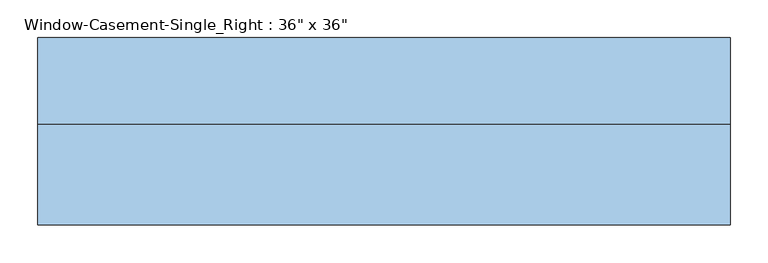
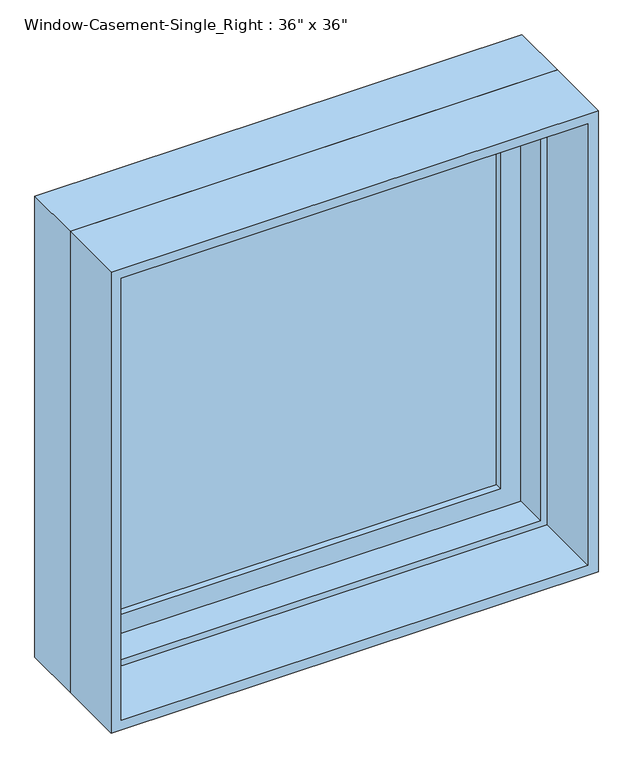
"""IFC4 building model written with IfcOpenShell, lengths in millimetres: window geometry."""

from ifc_helpers import new_model, si_unit, frame, origin, place, context, project, spatial, polyline, outline, extrude, faceted_brep, source, transform, mapped, element, save


def window_df0b8b67(model_context):
    return source(origin(), model_context, "Body", "SolidModel", [
        faceted_brep([(425.45, 82.55, 1797.05), (425.45, 19.05, 1797.05), (-425.45, 19.05, 1797.05), (-425.45, 82.55, 1797.05), (444.5, 133.35, 1816.1), (444.5, 82.55, 1816.1), (-444.5, 82.55, 1816.1), (-444.5, 133.35, 1816.1), (457.2, 19.05, 1828.8), (457.2, 133.35, 1828.8), (-457.2, 133.35, 1828.8), (-457.2, 19.05, 1828.8), (-425.45, 19.05, 946.15), (-425.45, 82.55, 946.15), (-444.5, 82.55, 927.1), (-444.5, 133.35, 927.1), (-457.2, 133.35, 914.4), (-457.2, 19.05, 914.4), (425.45, 19.05, 946.15), (425.45, 82.55, 946.15), (444.5, 82.55, 927.1), (444.5, 133.35, 927.1), (457.2, 133.35, 914.4), (457.2, 19.05, 914.4)], [[[0, 1, 2, 3]], [[4, 5, 6, 7]], [[8, 9, 10, 11]], [[3, 2, 12, 13]], [[7, 6, 14, 15]], [[11, 10, 16, 17]], [[13, 12, 18, 19]], [[15, 14, 20, 21]], [[17, 16, 22, 23]], [[11, 17, 23, 8], [1, 18, 12, 2]], [[19, 18, 1, 0]], [[5, 20, 14, 6], [3, 13, 19, 0]], [[21, 20, 5, 4]], [[23, 22, 9, 8]], [[9, 22, 16, 10], [7, 15, 21, 4]]]),
        extrude(outline(polyline([(1828.8, -457.2), (914.4, -457.2), (914.4, 457.2), (1828.8, 457.2), (1828.8, -457.2)]), holes=[polyline([(1809.75, 438.15), (933.45, 438.15), (933.45, -438.15), (1809.75, -438.15), (1809.75, 438.15)])]), frame((0.0, -114.3, 0.0), z_axis=(0.0, 1.0, 0.0), x_axis=(0.0, 0.0, 1.0)), (0.0, 0.0, 1.0), 133.35),
        extrude(outline(polyline([(1816.1, -444.5), (927.1, -444.5), (927.1, 444.5), (1816.1, 444.5), (1816.1, -444.5)]), holes=[polyline([(1758.95, 387.35), (984.25, 387.35), (984.25, -387.35), (1758.95, -387.35), (1758.95, 387.35)])]), frame((0.0, 82.55, 0.0), z_axis=(0.0, 1.0, 0.0), x_axis=(0.0, 0.0, 1.0)), (0.0, 0.0, 1.0), 44.45),
        extrude(outline(polyline([(387.35, 114.3), (387.35, 107.95), (-387.35, 107.95), (-387.35, 114.3), (387.35, 114.3)])), frame((0.0, 0.0, 984.25), z_axis=(0.0, 0.0, 1.0), x_axis=(1.0, 0.0, 0.0)), (0.0, 0.0, 1.0), 774.7),
        extrude(outline(polyline([(-387.35, 95.25), (-387.35, 101.6), (387.35, 101.6), (387.35, 95.25), (-387.35, 95.25)])), frame((0.0, 0.0, 984.25), z_axis=(0.0, 0.0, 1.0), x_axis=(1.0, 0.0, 0.0)), (0.0, 0.0, 1.0), 774.7),
    ])


if __name__ == "__main__":
    model = new_model("IFC4")
    model_context = context("Model", 3, world=origin())
    ifc_project = project(units=[si_unit("LENGTHUNIT", "METRE", prefix="MILLI")], contexts=[model_context])
    site = spatial("IfcSite", under=ifc_project)
    building = spatial("IfcBuilding", under=site)
    placement = place(None, origin())
    window_shape = window_df0b8b67(model_context)
    element("IfcWindow", 1, ObjectType="Window-Casement-Single_Right : 36\" x 36\"", at=placement, inside=building, context=model_context, shape_type="MappedRepresentation", body=[
        mapped(window_shape, transform((0.0, 0.0, 0.0), x_axis=(1.0, 0.0, 0.0), y_axis=(0.0, 1.0, 0.0), z_axis=(0.0, 0.0, 1.0))),
    ])
    save(model, "model.ifc")

# Revit data of these elements
# Type "Window-Casement-Single_Right : 36\" x 36\""
#   Type Mark = "50"
#   Fire Rating = "0.5h"
#   Assembly Code = "B2020100"
#   Analytic Construction = "Double glazing - domestic"
#   Window Inset [instance default] = 0' - 0"
#   Wall Thickness [instance default] = 0' - 6"
#   Visual Light Transmittance = 0.81
#   Thermal Resistance (R) = 0.319569 (m²·K)/W
#   Solar Heat Gain Coefficient = 0.76
#   Rough Width = 3' - 0 1/2"
#   Rough Height = 3' - 0 1/2"
#   Interior Wall Closure [instance default] = 0' - 2 1/4"
#   Height = 3' - 0"
#   Heat Transfer Coefficient (U) = 3.12929 W/(m²·K)
#   Frame Extension [instance default] = 0' - 0 1/4"
#   Exterior Wall Closure [instance default] = 0' - 1 1/4"
#   Extension Jamb [instance default] = 0' - 2 1/4"
#   Default Sill Height = 3' - 0"
#   Width = 3' - 0"
#   Muntin Visibility = yes
#   Interior Trim Visibility [instance default] = yes
#   Exterior Trim Visibility [instance default] = yes
#   Extension Jamb Visibility [instance default] = yes
#   Muntin Pattern = Muntin Pattern_2x2 : Muntin Pattern_2x2
#   Interior Trim Material = Wood - Stained
#   Interior Trim = Trim-Window-Interior-Flat : Picture Frame
#   Interior Frame Material = Wood - Stained
#   Glass Panel Material = Glass
#   Exterior Trim Material = Clad - White
#   Exterior Trim = Trim-Window-Exterior-Flat : with Sill
#   Exterior Frame Material = Clad - White
#   Wall Closure = (empty or 0)
# Element 1 (IfcWindow, "Window-Casement-Single_Right : 36\" x 36\"")
#   Wall Thickness = 0' - 9"
#   Extension Jamb = 0' - 5 1/4"
#   Materials on its faces: "Wood - Stained", "Glass", "Clad - White"
# Materials
#   "Wood - Stained": class "Wood", colour RGB 227 170 128, transparency 0, Cost = 0
#   "Glass": class "Glass", colour RGB 0 128 192, transparency 0.9, Description = "Soda Lime Glass", Cost = 0
#   "Clad - White": class "Wood", colour RGB 242 242 238, transparency 0, Cost = 0
